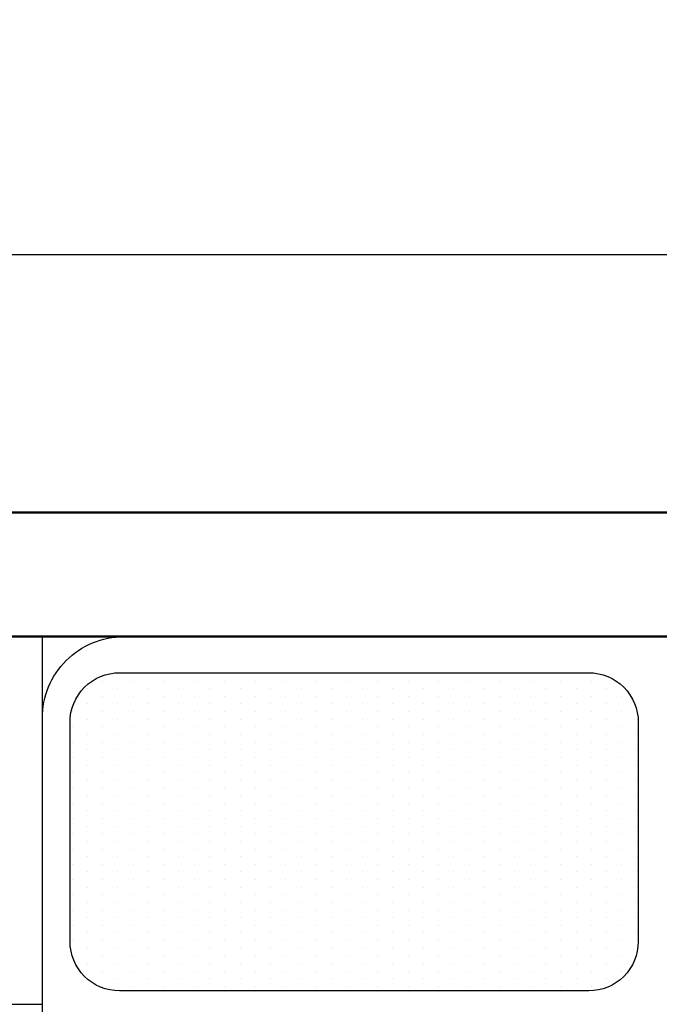
# Model space of a CAD drawing. Units: inches. Extents: x 3064 to 19385, y 846 to 15425.
# Tile 22 of 108: x 3855 to 3886, y 1373 to 1420. Entities that reach past the tile are written whole.
import ezdxf

# ---------------------------------------------------------------- set-up
doc = ezdxf.new("R2010")
doc.units = ezdxf.units.IN
for name, color, linetype, lineweight in [('A-ANNO-DIMS', 2, 'Continuous', 18), ('A-FLOR-FIXT', 9, 'Continuous', 18), ('A-WALL', 7, 'Continuous', 50)]:
    doc.layers.add(name, color=color, linetype=linetype, lineweight=lineweight)
doc.layers.add('BLOCK', color=6, linetype='Continuous')
doc.styles.get("Standard").update_dxf_attribs({"font": 'arial.ttf'})
doc.dimstyles.new('ISO-25', dxfattribs={"dimtxt": 9, "dimasz": 2.5, "dimexe": 1.25, "dimexo": 0.625, "dimtad": 1, "dimdec": 1, "dimlunit": 3, "dimtxsty": 'Standard', "dimcen": 2.5, "dimadec": 0, "dimazin": 0, "dimtfac": 1, "dimtdec": 1, "dimtmove": 0, "dimatfit": 3, "dimfxl": 1, "dimarcsym": 0})

# ---------------------------------------------------------------- blocks, each defined once
blk = doc.blocks.new('*X7')
at = {"color": 0}
for p, q in [((266.4375, 457.03125), (266.4375, 457.03125)), ((266.8125, 457.03125), (266.8125, 457.03125)), ((267.1875, 457.03125), (267.1875, 457.03125)), ((267.5625, 457.03125), (267.5625, 457.03125)), ((267.9375, 457.03125), (267.9375, 457.03125)), ((268.3125, 457.03125), (268.3125, 457.03125)), ((268.6875, 457.03125), (268.6875, 457.03125)), ((269.0625, 457.03125), (269.0625, 457.03125)), ((269.4375, 457.03125), (269.4375, 457.03125)), ((269.8125, 457.03125), (269.8125, 457.03125)), ((270.1875, 457.03125), (270.1875, 457.03125)), ((270.5625, 457.03125), (270.5625, 457.03125)), ((270.9375, 457.03125), (270.9375, 457.03125)), ((271.3125, 457.03125), (271.3125, 457.03125)), ((271.6875, 457.03125), (271.6875, 457.03125)), ((272.0625, 457.03125), (272.0625, 457.03125)), ((266.0625, 456.84375), (266.0625, 456.84375)), ((266.25, 456.9375), (266.25, 456.9375)), ((266.4375, 456.84375), (266.4375, 456.84375)), ((266.625, 456.9375), (266.625, 456.9375)), ((266.8125, 456.84375), (266.8125, 456.84375)), ((267, 456.9375), (267, 456.9375)), ((267.1875, 456.84375), (267.1875, 456.84375)), ((267.375, 456.9375), (267.375, 456.9375)), ((267.5625, 456.84375), (267.5625, 456.84375)), ((267.75, 456.9375), (267.75, 456.9375)), ((267.9375, 456.84375), (267.9375, 456.84375)), ((268.125, 456.9375), (268.125, 456.9375)), ((268.3125, 456.84375), (268.3125, 456.84375)), ((268.5, 456.9375), (268.5, 456.9375)), ((268.6875, 456.84375), (268.6875, 456.84375)), ((268.875, 456.9375), (268.875, 456.9375)), ((269.0625, 456.84375), (269.0625, 456.84375)), ((269.25, 456.9375), (269.25, 456.9375)), ((269.4375, 456.84375), (269.4375, 456.84375)), ((269.625, 456.9375), (269.625, 456.9375)), ((269.8125, 456.84375), (269.8125, 456.84375)), ((270, 456.9375), (270, 456.9375)), ((270.1875, 456.84375), (270.1875, 456.84375)), ((270.375, 456.9375), (270.375, 456.9375)), ((270.5625, 456.84375), (270.5625, 456.84375)), ((270.75, 456.9375), (270.75, 456.9375)), ((270.9375, 456.84375), (270.9375, 456.84375)), ((271.125, 456.9375), (271.125, 456.9375)), ((271.3125, 456.84375), (271.3125, 456.84375)), ((271.5, 456.9375), (271.5, 456.9375)), ((271.6875, 456.84375), (271.6875, 456.84375)), ((271.875, 456.9375), (271.875, 456.9375)), ((272.0625, 456.84375), (272.0625, 456.84375)), ((272.25, 456.9375), (272.25, 456.9375)), ((272.4375, 456.84375), (272.4375, 456.84375)), ((266.25, 456.75), (266.25, 456.75)), ((266.625, 456.75), (266.625, 456.75)), ((267, 456.75), (267, 456.75)), ((267.375, 456.75), (267.375, 456.75)), ((267.75, 456.75), (267.75, 456.75)), ((268.125, 456.75), (268.125, 456.75)), ((268.5, 456.75), (268.5, 456.75)), ((268.875, 456.75), (268.875, 456.75)), ((269.25, 456.75), (269.25, 456.75)), ((269.625, 456.75), (269.625, 456.75)), ((270, 456.75), (270, 456.75)), ((270.375, 456.75), (270.375, 456.75)), ((270.75, 456.75), (270.75, 456.75)), ((271.125, 456.75), (271.125, 456.75)), ((271.5, 456.75), (271.5, 456.75)), ((271.875, 456.75), (271.875, 456.75)), ((272.25, 456.75), (272.25, 456.75)), ((272.625, 456.75), (272.625, 456.75)), ((266.0625, 456.65625), (266.0625, 456.65625)), ((266.4375, 456.65625), (266.4375, 456.65625)), ((266.8125, 456.65625), (266.8125, 456.65625)), ((267.1875, 456.65625), (267.1875, 456.65625)), ((267.5625, 456.65625), (267.5625, 456.65625)), ((267.9375, 456.65625), (267.9375, 456.65625)), ((268.3125, 456.65625), (268.3125, 456.65625)), ((268.6875, 456.65625), (268.6875, 456.65625)), ((269.0625, 456.65625), (269.0625, 456.65625)), ((269.4375, 456.65625), (269.4375, 456.65625)), ((269.8125, 456.65625), (269.8125, 456.65625)), ((270.1875, 456.65625), (270.1875, 456.65625)), ((270.5625, 456.65625), (270.5625, 456.65625)), ((270.9375, 456.65625), (270.9375, 456.65625)), ((271.3125, 456.65625), (271.3125, 456.65625)), ((271.6875, 456.65625), (271.6875, 456.65625)), ((272.0625, 456.65625), (272.0625, 456.65625)), ((272.4375, 456.65625), (272.4375, 456.65625)), ((265.875, 456.5625), (265.875, 456.5625)), ((266.25, 456.5625), (266.25, 456.5625)), ((266.625, 456.5625), (266.625, 456.5625)), ((267, 456.5625), (267, 456.5625)), ((267.375, 456.5625), (267.375, 456.5625)), ((267.75, 456.5625), (267.75, 456.5625)), ((268.125, 456.5625), (268.125, 456.5625)), ((268.5, 456.5625), (268.5, 456.5625)), ((268.875, 456.5625), (268.875, 456.5625)), ((269.25, 456.5625), (269.25, 456.5625)), ((269.625, 456.5625), (269.625, 456.5625)), ((270, 456.5625), (270, 456.5625)), ((270.375, 456.5625), (270.375, 456.5625)), ((270.75, 456.5625), (270.75, 456.5625)), ((271.125, 456.5625), (271.125, 456.5625)), ((271.5, 456.5625), (271.5, 456.5625)), ((271.875, 456.5625), (271.875, 456.5625)), ((272.25, 456.5625), (272.25, 456.5625)), ((272.625, 456.5625), (272.625, 456.5625)), ((265.875, 456.375), (265.875, 456.375)), ((266.0625, 456.46875), (266.0625, 456.46875)), ((266.25, 456.375), (266.25, 456.375)), ((266.4375, 456.46875), (266.4375, 456.46875)), ((266.625, 456.375), (266.625, 456.375)), ((266.8125, 456.46875), (266.8125, 456.46875)), ((267, 456.375), (267, 456.375)), ((267.1875, 456.46875), (267.1875, 456.46875)), ((267.375, 456.375), (267.375, 456.375)), ((267.5625, 456.46875), (267.5625, 456.46875)), ((267.75, 456.375), (267.75, 456.375)), ((267.9375, 456.46875), (267.9375, 456.46875)), ((268.125, 456.375), (268.125, 456.375)), ((268.3125, 456.46875), (268.3125, 456.46875)), ((268.5, 456.375), (268.5, 456.375)), ((268.6875, 456.46875), (268.6875, 456.46875)), ((268.875, 456.375), (268.875, 456.375)), ((269.0625, 456.46875), (269.0625, 456.46875)), ((269.25, 456.375), (269.25, 456.375)), ((269.4375, 456.46875), (269.4375, 456.46875)), ((269.625, 456.375), (269.625, 456.375)), ((269.8125, 456.46875), (269.8125, 456.46875)), ((270, 456.375), (270, 456.375)), ((270.1875, 456.46875), (270.1875, 456.46875)), ((270.375, 456.375), (270.375, 456.375)), ((270.5625, 456.46875), (270.5625, 456.46875)), ((270.75, 456.375), (270.75, 456.375)), ((270.9375, 456.46875), (270.9375, 456.46875)), ((271.125, 456.375), (271.125, 456.375)), ((271.3125, 456.46875), (271.3125, 456.46875)), ((271.5, 456.375), (271.5, 456.375)), ((271.6875, 456.46875), (271.6875, 456.46875)), ((271.875, 456.375), (271.875, 456.375)), ((272.0625, 456.46875), (272.0625, 456.46875)), ((272.25, 456.375), (272.25, 456.375)), ((272.4375, 456.46875), (272.4375, 456.46875)), ((272.625, 456.375), (272.625, 456.375)), ((272.8125, 456.46875), (272.8125, 456.46875)), ((266.0625, 456.28125), (266.0625, 456.28125)), ((266.4375, 456.28125), (266.4375, 456.28125)), ((266.8125, 456.28125), (266.8125, 456.28125)), ((267.1875, 456.28125), (267.1875, 456.28125)), ((267.5625, 456.28125), (267.5625, 456.28125)), ((267.9375, 456.28125), (267.9375, 456.28125)), ((268.3125, 456.28125), (268.3125, 456.28125)), ((268.6875, 456.28125), (268.6875, 456.28125)), ((269.0625, 456.28125), (269.0625, 456.28125)), ((269.4375, 456.28125), (269.4375, 456.28125)), ((269.8125, 456.28125), (269.8125, 456.28125)), ((270.1875, 456.28125), (270.1875, 456.28125)), ((270.5625, 456.28125), (270.5625, 456.28125)), ((270.9375, 456.28125), (270.9375, 456.28125)), ((271.3125, 456.28125), (271.3125, 456.28125)), ((271.6875, 456.28125), (271.6875, 456.28125)), ((272.0625, 456.28125), (272.0625, 456.28125)), ((272.4375, 456.28125), (272.4375, 456.28125)), ((272.8125, 456.28125), (272.8125, 456.28125)), ((265.875, 456.1875), (265.875, 456.1875)), ((266.25, 456.1875), (266.25, 456.1875)), ((266.625, 456.1875), (266.625, 456.1875)), ((267, 456.1875), (267, 456.1875)), ((267.375, 456.1875), (267.375, 456.1875)), ((267.75, 456.1875), (267.75, 456.1875)), ((268.125, 456.1875), (268.125, 456.1875)), ((268.5, 456.1875), (268.5, 456.1875)), ((268.875, 456.1875), (268.875, 456.1875)), ((269.25, 456.1875), (269.25, 456.1875)), ((269.625, 456.1875), (269.625, 456.1875)), ((270, 456.1875), (270, 456.1875)), ((270.375, 456.1875), (270.375, 456.1875)), ((270.75, 456.1875), (270.75, 456.1875)), ((271.125, 456.1875), (271.125, 456.1875)), ((271.5, 456.1875), (271.5, 456.1875)), ((271.875, 456.1875), (271.875, 456.1875)), ((272.25, 456.1875), (272.25, 456.1875)), ((272.625, 456.1875), (272.625, 456.1875)), ((265.875, 456), (265.875, 456)), ((266.0625, 456.09375), (266.0625, 456.09375)), ((266.25, 456), (266.25, 456)), ((266.4375, 456.09375), (266.4375, 456.09375)), ((266.625, 456), (266.625, 456)), ((266.8125, 456.09375), (266.8125, 456.09375)), ((267, 456), (267, 456)), ((267.1875, 456.09375), (267.1875, 456.09375)), ((267.375, 456), (267.375, 456)), ((267.5625, 456.09375), (267.5625, 456.09375)), ((267.75, 456), (267.75, 456)), ((267.9375, 456.09375), (267.9375, 456.09375)), ((268.125, 456), (268.125, 456)), ((268.3125, 456.09375), (268.3125, 456.09375)), ((268.5, 456), (268.5, 456)), ((268.6875, 456.09375), (268.6875, 456.09375)), ((268.875, 456), (268.875, 456)), ((269.0625, 456.09375), (269.0625, 456.09375)), ((269.25, 456), (269.25, 456)), ((269.4375, 456.09375), (269.4375, 456.09375)), ((269.625, 456), (269.625, 456)), ((269.8125, 456.09375), (269.8125, 456.09375)), ((270, 456), (270, 456)), ((270.1875, 456.09375), (270.1875, 456.09375)), ((270.375, 456), (270.375, 456)), ((270.5625, 456.09375), (270.5625, 456.09375)), ((270.75, 456), (270.75, 456)), ((270.9375, 456.09375), (270.9375, 456.09375)), ((271.125, 456), (271.125, 456)), ((271.3125, 456.09375), (271.3125, 456.09375)), ((271.5, 456), (271.5, 456)), ((271.6875, 456.09375), (271.6875, 456.09375)), ((271.875, 456), (271.875, 456)), ((272.0625, 456.09375), (272.0625, 456.09375)), ((272.25, 456), (272.25, 456)), ((272.4375, 456.09375), (272.4375, 456.09375)), ((272.625, 456), (272.625, 456)), ((272.8125, 456.09375), (272.8125, 456.09375)), ((266.0625, 455.90625), (266.0625, 455.90625)), ((266.4375, 455.90625), (266.4375, 455.90625)), ((266.8125, 455.90625), (266.8125, 455.90625)), ((267.1875, 455.90625), (267.1875, 455.90625)), ((267.5625, 455.90625), (267.5625, 455.90625)), ((267.9375, 455.90625), (267.9375, 455.90625)), ((268.3125, 455.90625), (268.3125, 455.90625)), ((268.6875, 455.90625), (268.6875, 455.90625)), ((269.0625, 455.90625), (269.0625, 455.90625)), ((269.4375, 455.90625), (269.4375, 455.90625)), ((269.8125, 455.90625), (269.8125, 455.90625)), ((270.1875, 455.90625), (270.1875, 455.90625)), ((270.5625, 455.90625), (270.5625, 455.90625)), ((270.9375, 455.90625), (270.9375, 455.90625)), ((271.3125, 455.90625), (271.3125, 455.90625)), ((271.6875, 455.90625), (271.6875, 455.90625)), ((272.0625, 455.90625), (272.0625, 455.90625)), ((272.4375, 455.90625), (272.4375, 455.90625)), ((272.8125, 455.90625), (272.8125, 455.90625)), ((265.875, 455.8125), (265.875, 455.8125)), ((266.25, 455.8125), (266.25, 455.8125)), ((266.625, 455.8125), (266.625, 455.8125)), ((267, 455.8125), (267, 455.8125)), ((267.375, 455.8125), (267.375, 455.8125)), ((267.75, 455.8125), (267.75, 455.8125)), ((268.125, 455.8125), (268.125, 455.8125)), ((268.5, 455.8125), (268.5, 455.8125)), ((268.875, 455.8125), (268.875, 455.8125)), ((269.25, 455.8125), (269.25, 455.8125)), ((269.625, 455.8125), (269.625, 455.8125)), ((270, 455.8125), (270, 455.8125)), ((270.375, 455.8125), (270.375, 455.8125)), ((270.75, 455.8125), (270.75, 455.8125)), ((271.125, 455.8125), (271.125, 455.8125)), ((271.5, 455.8125), (271.5, 455.8125)), ((271.875, 455.8125), (271.875, 455.8125)), ((272.25, 455.8125), (272.25, 455.8125)), ((272.625, 455.8125), (272.625, 455.8125)), ((265.875, 455.625), (265.875, 455.625)), ((266.0625, 455.71875), (266.0625, 455.71875)), ((266.25, 455.625), (266.25, 455.625)), ((266.4375, 455.71875), (266.4375, 455.71875)), ((266.625, 455.625), (266.625, 455.625)), ((266.8125, 455.71875), (266.8125, 455.71875)), ((267, 455.625), (267, 455.625)), ((267.1875, 455.71875), (267.1875, 455.71875)), ((267.375, 455.625), (267.375, 455.625)), ((267.5625, 455.71875), (267.5625, 455.71875)), ((267.75, 455.625), (267.75, 455.625)), ((267.9375, 455.71875), (267.9375, 455.71875)), ((268.125, 455.625), (268.125, 455.625)), ((268.3125, 455.71875), (268.3125, 455.71875)), ((268.5, 455.625), (268.5, 455.625)), ((268.6875, 455.71875), (268.6875, 455.71875)), ((268.875, 455.625), (268.875, 455.625)), ((269.0625, 455.71875), (269.0625, 455.71875)), ((269.25, 455.625), (269.25, 455.625)), ((269.4375, 455.71875), (269.4375, 455.71875)), ((269.625, 455.625), (269.625, 455.625)), ((269.8125, 455.71875), (269.8125, 455.71875)), ((270, 455.625), (270, 455.625)), ((270.1875, 455.71875), (270.1875, 455.71875)), ((270.375, 455.625), (270.375, 455.625)), ((270.5625, 455.71875), (270.5625, 455.71875)), ((270.75, 455.625), (270.75, 455.625)), ((270.9375, 455.71875), (270.9375, 455.71875)), ((271.125, 455.625), (271.125, 455.625)), ((271.3125, 455.71875), (271.3125, 455.71875)), ((271.5, 455.625), (271.5, 455.625)), ((271.6875, 455.71875), (271.6875, 455.71875)), ((271.875, 455.625), (271.875, 455.625)), ((272.0625, 455.71875), (272.0625, 455.71875)), ((272.25, 455.625), (272.25, 455.625)), ((272.4375, 455.71875), (272.4375, 455.71875)), ((272.625, 455.625), (272.625, 455.625)), ((272.8125, 455.71875), (272.8125, 455.71875)), ((266.0625, 455.53125), (266.0625, 455.53125)), ((266.4375, 455.53125), (266.4375, 455.53125)), ((266.8125, 455.53125), (266.8125, 455.53125)), ((267.1875, 455.53125), (267.1875, 455.53125)), ((267.5625, 455.53125), (267.5625, 455.53125)), ((267.9375, 455.53125), (267.9375, 455.53125)), ((268.3125, 455.53125), (268.3125, 455.53125)), ((268.6875, 455.53125), (268.6875, 455.53125)), ((269.0625, 455.53125), (269.0625, 455.53125)), ((269.4375, 455.53125), (269.4375, 455.53125)), ((269.8125, 455.53125), (269.8125, 455.53125)), ((270.1875, 455.53125), (270.1875, 455.53125)), ((270.5625, 455.53125), (270.5625, 455.53125)), ((270.9375, 455.53125), (270.9375, 455.53125)), ((271.3125, 455.53125), (271.3125, 455.53125)), ((271.6875, 455.53125), (271.6875, 455.53125)), ((272.0625, 455.53125), (272.0625, 455.53125)), ((272.4375, 455.53125), (272.4375, 455.53125)), ((272.8125, 455.53125), (272.8125, 455.53125)), ((265.875, 455.4375), (265.875, 455.4375)), ((266.25, 455.4375), (266.25, 455.4375)), ((266.625, 455.4375), (266.625, 455.4375)), ((267, 455.4375), (267, 455.4375)), ((267.375, 455.4375), (267.375, 455.4375)), ((267.75, 455.4375), (267.75, 455.4375)), ((268.125, 455.4375), (268.125, 455.4375)), ((268.5, 455.4375), (268.5, 455.4375)), ((268.875, 455.4375), (268.875, 455.4375)), ((269.25, 455.4375), (269.25, 455.4375)), ((269.625, 455.4375), (269.625, 455.4375)), ((270, 455.4375), (270, 455.4375)), ((270.375, 455.4375), (270.375, 455.4375)), ((270.75, 455.4375), (270.75, 455.4375)), ((271.125, 455.4375), (271.125, 455.4375)), ((271.5, 455.4375), (271.5, 455.4375)), ((271.875, 455.4375), (271.875, 455.4375)), ((272.25, 455.4375), (272.25, 455.4375)), ((272.625, 455.4375), (272.625, 455.4375)), ((266.0625, 455.34375), (266.0625, 455.34375)), ((266.4375, 455.34375), (266.4375, 455.34375)), ((266.8125, 455.34375), (266.8125, 455.34375)), ((267.1875, 455.34375), (267.1875, 455.34375)), ((267.5625, 455.34375), (267.5625, 455.34375)), ((267.9375, 455.34375), (267.9375, 455.34375)), ((268.3125, 455.34375), (268.3125, 455.34375)), ((268.6875, 455.34375), (268.6875, 455.34375)), ((269.0625, 455.34375), (269.0625, 455.34375)), ((269.4375, 455.34375), (269.4375, 455.34375)), ((269.8125, 455.34375), (269.8125, 455.34375)), ((270.1875, 455.34375), (270.1875, 455.34375)), ((270.5625, 455.34375), (270.5625, 455.34375)), ((270.9375, 455.34375), (270.9375, 455.34375)), ((271.3125, 455.34375), (271.3125, 455.34375)), ((271.6875, 455.34375), (271.6875, 455.34375)), ((272.0625, 455.34375), (272.0625, 455.34375)), ((272.4375, 455.34375), (272.4375, 455.34375)), ((272.8125, 455.34375), (272.8125, 455.34375)), ((265.875, 455.25), (265.875, 455.25)), ((266.0625, 455.15625), (266.0625, 455.15625)), ((266.25, 455.25), (266.25, 455.25)), ((266.4375, 455.15625), (266.4375, 455.15625)), ((266.625, 455.25), (266.625, 455.25)), ((266.8125, 455.15625), (266.8125, 455.15625)), ((267, 455.25), (267, 455.25)), ((267.1875, 455.15625), (267.1875, 455.15625)), ((267.375, 455.25), (267.375, 455.25)), ((267.5625, 455.15625), (267.5625, 455.15625)), ((267.75, 455.25), (267.75, 455.25)), ((267.9375, 455.15625), (267.9375, 455.15625)), ((268.125, 455.25), (268.125, 455.25)), ((268.3125, 455.15625), (268.3125, 455.15625)), ((268.5, 455.25), (268.5, 455.25)), ((268.6875, 455.15625), (268.6875, 455.15625)), ((268.875, 455.25), (268.875, 455.25)), ((269.0625, 455.15625), (269.0625, 455.15625)), ((269.25, 455.25), (269.25, 455.25)), ((269.4375, 455.15625), (269.4375, 455.15625)), ((269.625, 455.25), (269.625, 455.25)), ((269.8125, 455.15625), (269.8125, 455.15625)), ((270, 455.25), (270, 455.25)), ((270.1875, 455.15625), (270.1875, 455.15625)), ((270.375, 455.25), (270.375, 455.25)), ((270.5625, 455.15625), (270.5625, 455.15625)), ((270.75, 455.25), (270.75, 455.25)), ((270.9375, 455.15625), (270.9375, 455.15625)), ((271.125, 455.25), (271.125, 455.25)), ((271.3125, 455.15625), (271.3125, 455.15625)), ((271.5, 455.25), (271.5, 455.25)), ((271.6875, 455.15625), (271.6875, 455.15625)), ((271.875, 455.25), (271.875, 455.25)), ((272.0625, 455.15625), (272.0625, 455.15625)), ((272.25, 455.25), (272.25, 455.25)), ((272.4375, 455.15625), (272.4375, 455.15625)), ((272.625, 455.25), (272.625, 455.25)), ((272.8125, 455.15625), (272.8125, 455.15625)), ((265.875, 455.0625), (265.875, 455.0625)), ((266.25, 455.0625), (266.25, 455.0625)), ((266.625, 455.0625), (266.625, 455.0625)), ((267, 455.0625), (267, 455.0625)), ((267.375, 455.0625), (267.375, 455.0625)), ((267.75, 455.0625), (267.75, 455.0625)), ((268.125, 455.0625), (268.125, 455.0625)), ((268.5, 455.0625), (268.5, 455.0625)), ((268.875, 455.0625), (268.875, 455.0625)), ((269.25, 455.0625), (269.25, 455.0625)), ((269.625, 455.0625), (269.625, 455.0625)), ((270, 455.0625), (270, 455.0625)), ((270.375, 455.0625), (270.375, 455.0625)), ((270.75, 455.0625), (270.75, 455.0625)), ((271.125, 455.0625), (271.125, 455.0625)), ((271.5, 455.0625), (271.5, 455.0625)), ((271.875, 455.0625), (271.875, 455.0625)), ((272.25, 455.0625), (272.25, 455.0625)), ((272.625, 455.0625), (272.625, 455.0625)), ((266.0625, 454.96875), (266.0625, 454.96875)), ((266.4375, 454.96875), (266.4375, 454.96875)), ((266.8125, 454.96875), (266.8125, 454.96875)), ((267.1875, 454.96875), (267.1875, 454.96875)), ((267.5625, 454.96875), (267.5625, 454.96875)), ((267.9375, 454.96875), (267.9375, 454.96875)), ((268.3125, 454.96875), (268.3125, 454.96875)), ((268.6875, 454.96875), (268.6875, 454.96875)), ((269.0625, 454.96875), (269.0625, 454.96875)), ((269.4375, 454.96875), (269.4375, 454.96875)), ((269.8125, 454.96875), (269.8125, 454.96875)), ((270.1875, 454.96875), (270.1875, 454.96875)), ((270.5625, 454.96875), (270.5625, 454.96875)), ((270.9375, 454.96875), (270.9375, 454.96875)), ((271.3125, 454.96875), (271.3125, 454.96875)), ((271.6875, 454.96875), (271.6875, 454.96875)), ((272.0625, 454.96875), (272.0625, 454.96875)), ((272.4375, 454.96875), (272.4375, 454.96875)), ((272.8125, 454.96875), (272.8125, 454.96875)), ((265.875, 454.875), (265.875, 454.875)), ((266.0625, 454.78125), (266.0625, 454.78125)), ((266.25, 454.875), (266.25, 454.875)), ((266.4375, 454.78125), (266.4375, 454.78125)), ((266.625, 454.875), (266.625, 454.875)), ((266.8125, 454.78125), (266.8125, 454.78125)), ((267, 454.875), (267, 454.875)), ((267.1875, 454.78125), (267.1875, 454.78125)), ((267.375, 454.875), (267.375, 454.875)), ((267.5625, 454.78125), (267.5625, 454.78125)), ((267.75, 454.875), (267.75, 454.875)), ((267.9375, 454.78125), (267.9375, 454.78125)), ((268.125, 454.875), (268.125, 454.875)), ((268.3125, 454.78125), (268.3125, 454.78125)), ((268.5, 454.875), (268.5, 454.875)), ((268.6875, 454.78125), (268.6875, 454.78125)), ((268.875, 454.875), (268.875, 454.875)), ((269.0625, 454.78125), (269.0625, 454.78125)), ((269.25, 454.875), (269.25, 454.875)), ((269.4375, 454.78125), (269.4375, 454.78125)), ((269.625, 454.875), (269.625, 454.875)), ((269.8125, 454.78125), (269.8125, 454.78125)), ((270, 454.875), (270, 454.875)), ((270.1875, 454.78125), (270.1875, 454.78125)), ((270.375, 454.875), (270.375, 454.875)), ((270.5625, 454.78125), (270.5625, 454.78125)), ((270.75, 454.875), (270.75, 454.875)), ((270.9375, 454.78125), (270.9375, 454.78125)), ((271.125, 454.875), (271.125, 454.875)), ((271.3125, 454.78125), (271.3125, 454.78125)), ((271.5, 454.875), (271.5, 454.875)), ((271.6875, 454.78125), (271.6875, 454.78125)), ((271.875, 454.875), (271.875, 454.875)), ((272.0625, 454.78125), (272.0625, 454.78125)), ((272.25, 454.875), (272.25, 454.875)), ((272.4375, 454.78125), (272.4375, 454.78125)), ((272.625, 454.875), (272.625, 454.875)), ((272.8125, 454.78125), (272.8125, 454.78125)), ((265.875, 454.6875), (265.875, 454.6875)), ((266.25, 454.6875), (266.25, 454.6875)), ((266.625, 454.6875), (266.625, 454.6875)), ((267, 454.6875), (267, 454.6875)), ((267.375, 454.6875), (267.375, 454.6875)), ((267.75, 454.6875), (267.75, 454.6875)), ((268.125, 454.6875), (268.125, 454.6875)), ((268.5, 454.6875), (268.5, 454.6875)), ((268.875, 454.6875), (268.875, 454.6875)), ((269.25, 454.6875), (269.25, 454.6875)), ((269.625, 454.6875), (269.625, 454.6875)), ((270, 454.6875), (270, 454.6875)), ((270.375, 454.6875), (270.375, 454.6875)), ((270.75, 454.6875), (270.75, 454.6875)), ((271.125, 454.6875), (271.125, 454.6875)), ((271.5, 454.6875), (271.5, 454.6875)), ((271.875, 454.6875), (271.875, 454.6875)), ((272.25, 454.6875), (272.25, 454.6875)), ((272.625, 454.6875), (272.625, 454.6875)), ((266.0625, 454.59375), (266.0625, 454.59375)), ((266.4375, 454.59375), (266.4375, 454.59375)), ((266.8125, 454.59375), (266.8125, 454.59375)), ((267.1875, 454.59375), (267.1875, 454.59375)), ((267.5625, 454.59375), (267.5625, 454.59375)), ((267.9375, 454.59375), (267.9375, 454.59375)), ((268.3125, 454.59375), (268.3125, 454.59375)), ((268.6875, 454.59375), (268.6875, 454.59375)), ((269.0625, 454.59375), (269.0625, 454.59375)), ((269.4375, 454.59375), (269.4375, 454.59375)), ((269.8125, 454.59375), (269.8125, 454.59375)), ((270.1875, 454.59375), (270.1875, 454.59375)), ((270.5625, 454.59375), (270.5625, 454.59375)), ((270.9375, 454.59375), (270.9375, 454.59375)), ((271.3125, 454.59375), (271.3125, 454.59375)), ((271.6875, 454.59375), (271.6875, 454.59375)), ((272.0625, 454.59375), (272.0625, 454.59375)), ((272.4375, 454.59375), (272.4375, 454.59375)), ((272.8125, 454.59375), (272.8125, 454.59375)), ((265.875, 454.5), (265.875, 454.5)), ((266.25, 454.5), (266.25, 454.5)), ((266.625, 454.5), (266.625, 454.5)), ((267, 454.5), (267, 454.5)), ((267.375, 454.5), (267.375, 454.5)), ((267.75, 454.5), (267.75, 454.5)), ((268.125, 454.5), (268.125, 454.5)), ((268.5, 454.5), (268.5, 454.5)), ((268.875, 454.5), (268.875, 454.5)), ((269.25, 454.5), (269.25, 454.5)), ((269.625, 454.5), (269.625, 454.5)), ((270, 454.5), (270, 454.5)), ((270.375, 454.5), (270.375, 454.5)), ((270.75, 454.5), (270.75, 454.5)), ((271.125, 454.5), (271.125, 454.5)), ((271.5, 454.5), (271.5, 454.5)), ((271.875, 454.5), (271.875, 454.5)), ((272.25, 454.5), (272.25, 454.5)), ((272.625, 454.5), (272.625, 454.5)), ((265.875, 454.3125), (265.875, 454.3125)), ((266.0625, 454.40625), (266.0625, 454.40625)), ((266.25, 454.3125), (266.25, 454.3125)), ((266.4375, 454.40625), (266.4375, 454.40625)), ((266.625, 454.3125), (266.625, 454.3125)), ((266.8125, 454.40625), (266.8125, 454.40625)), ((267, 454.3125), (267, 454.3125)), ((267.1875, 454.40625), (267.1875, 454.40625)), ((267.375, 454.3125), (267.375, 454.3125)), ((267.5625, 454.40625), (267.5625, 454.40625)), ((267.75, 454.3125), (267.75, 454.3125)), ((267.9375, 454.40625), (267.9375, 454.40625)), ((268.125, 454.3125), (268.125, 454.3125)), ((268.3125, 454.40625), (268.3125, 454.40625)), ((268.5, 454.3125), (268.5, 454.3125)), ((268.6875, 454.40625), (268.6875, 454.40625)), ((268.875, 454.3125), (268.875, 454.3125)), ((269.0625, 454.40625), (269.0625, 454.40625)), ((269.25, 454.3125), (269.25, 454.3125)), ((269.4375, 454.40625), (269.4375, 454.40625)), ((269.625, 454.3125), (269.625, 454.3125)), ((269.8125, 454.40625), (269.8125, 454.40625)), ((270, 454.3125), (270, 454.3125)), ((270.1875, 454.40625), (270.1875, 454.40625)), ((270.375, 454.3125), (270.375, 454.3125)), ((270.5625, 454.40625), (270.5625, 454.40625)), ((270.75, 454.3125), (270.75, 454.3125)), ((270.9375, 454.40625), (270.9375, 454.40625)), ((271.125, 454.3125), (271.125, 454.3125)), ((271.3125, 454.40625), (271.3125, 454.40625)), ((271.5, 454.3125), (271.5, 454.3125)), ((271.6875, 454.40625), (271.6875, 454.40625)), ((271.875, 454.3125), (271.875, 454.3125)), ((272.0625, 454.40625), (272.0625, 454.40625)), ((272.25, 454.3125), (272.25, 454.3125)), ((272.4375, 454.40625), (272.4375, 454.40625)), ((272.625, 454.3125), (272.625, 454.3125)), ((272.8125, 454.40625), (272.8125, 454.40625)), ((266.0625, 454.21875), (266.0625, 454.21875)), ((266.4375, 454.21875), (266.4375, 454.21875)), ((266.8125, 454.21875), (266.8125, 454.21875)), ((267.1875, 454.21875), (267.1875, 454.21875)), ((267.5625, 454.21875), (267.5625, 454.21875)), ((267.9375, 454.21875), (267.9375, 454.21875)), ((268.3125, 454.21875), (268.3125, 454.21875)), ((268.6875, 454.21875), (268.6875, 454.21875)), ((269.0625, 454.21875), (269.0625, 454.21875)), ((269.4375, 454.21875), (269.4375, 454.21875)), ((269.8125, 454.21875), (269.8125, 454.21875)), ((270.1875, 454.21875), (270.1875, 454.21875)), ((270.5625, 454.21875), (270.5625, 454.21875)), ((270.9375, 454.21875), (270.9375, 454.21875)), ((271.3125, 454.21875), (271.3125, 454.21875)), ((271.6875, 454.21875), (271.6875, 454.21875)), ((272.0625, 454.21875), (272.0625, 454.21875)), ((272.4375, 454.21875), (272.4375, 454.21875)), ((272.8125, 454.21875), (272.8125, 454.21875)), ((265.875, 454.125), (265.875, 454.125)), ((266.25, 454.125), (266.25, 454.125)), ((266.625, 454.125), (266.625, 454.125)), ((267, 454.125), (267, 454.125)), ((267.375, 454.125), (267.375, 454.125)), ((267.75, 454.125), (267.75, 454.125)), ((268.125, 454.125), (268.125, 454.125)), ((268.5, 454.125), (268.5, 454.125)), ((268.875, 454.125), (268.875, 454.125)), ((269.25, 454.125), (269.25, 454.125)), ((269.625, 454.125), (269.625, 454.125)), ((270, 454.125), (270, 454.125)), ((270.375, 454.125), (270.375, 454.125)), ((270.75, 454.125), (270.75, 454.125)), ((271.125, 454.125), (271.125, 454.125)), ((271.5, 454.125), (271.5, 454.125)), ((271.875, 454.125), (271.875, 454.125)), ((272.25, 454.125), (272.25, 454.125)), ((272.625, 454.125), (272.625, 454.125)), ((265.875, 453.9375), (265.875, 453.9375)), ((266.0625, 454.03125), (266.0625, 454.03125)), ((266.25, 453.9375), (266.25, 453.9375)), ((266.4375, 454.03125), (266.4375, 454.03125)), ((266.625, 453.9375), (266.625, 453.9375)), ((266.8125, 454.03125), (266.8125, 454.03125)), ((267, 453.9375), (267, 453.9375)), ((267.1875, 454.03125), (267.1875, 454.03125)), ((267.375, 453.9375), (267.375, 453.9375)), ((267.5625, 454.03125), (267.5625, 454.03125)), ((267.75, 453.9375), (267.75, 453.9375)), ((267.9375, 454.03125), (267.9375, 454.03125)), ((268.125, 453.9375), (268.125, 453.9375)), ((268.3125, 454.03125), (268.3125, 454.03125)), ((268.5, 453.9375), (268.5, 453.9375)), ((268.6875, 454.03125), (268.6875, 454.03125)), ((268.875, 453.9375), (268.875, 453.9375)), ((269.0625, 454.03125), (269.0625, 454.03125)), ((269.25, 453.9375), (269.25, 453.9375)), ((269.4375, 454.03125), (269.4375, 454.03125)), ((269.625, 453.9375), (269.625, 453.9375)), ((269.8125, 454.03125), (269.8125, 454.03125)), ((270, 453.9375), (270, 453.9375)), ((270.1875, 454.03125), (270.1875, 454.03125)), ((270.375, 453.9375), (270.375, 453.9375)), ((270.5625, 454.03125), (270.5625, 454.03125)), ((270.75, 453.9375), (270.75, 453.9375)), ((270.9375, 454.03125), (270.9375, 454.03125)), ((271.125, 453.9375), (271.125, 453.9375)), ((271.3125, 454.03125), (271.3125, 454.03125)), ((271.5, 453.9375), (271.5, 453.9375)), ((271.6875, 454.03125), (271.6875, 454.03125)), ((271.875, 453.9375), (271.875, 453.9375)), ((272.0625, 454.03125), (272.0625, 454.03125)), ((272.25, 453.9375), (272.25, 453.9375)), ((272.4375, 454.03125), (272.4375, 454.03125)), ((272.625, 453.9375), (272.625, 453.9375)), ((272.8125, 454.03125), (272.8125, 454.03125)), ((266.0625, 453.84375), (266.0625, 453.84375)), ((266.4375, 453.84375), (266.4375, 453.84375)), ((266.8125, 453.84375), (266.8125, 453.84375)), ((267.1875, 453.84375), (267.1875, 453.84375)), ((267.5625, 453.84375), (267.5625, 453.84375)), ((267.9375, 453.84375), (267.9375, 453.84375)), ((268.3125, 453.84375), (268.3125, 453.84375)), ((268.6875, 453.84375), (268.6875, 453.84375)), ((269.0625, 453.84375), (269.0625, 453.84375)), ((269.4375, 453.84375), (269.4375, 453.84375)), ((269.8125, 453.84375), (269.8125, 453.84375)), ((270.1875, 453.84375), (270.1875, 453.84375)), ((270.5625, 453.84375), (270.5625, 453.84375)), ((270.9375, 453.84375), (270.9375, 453.84375)), ((271.3125, 453.84375), (271.3125, 453.84375)), ((271.6875, 453.84375), (271.6875, 453.84375)), ((272.0625, 453.84375), (272.0625, 453.84375)), ((272.4375, 453.84375), (272.4375, 453.84375)), ((272.8125, 453.84375), (272.8125, 453.84375)), ((265.875, 453.75), (265.875, 453.75)), ((266.25, 453.75), (266.25, 453.75)), ((266.625, 453.75), (266.625, 453.75)), ((267, 453.75), (267, 453.75)), ((267.375, 453.75), (267.375, 453.75)), ((267.75, 453.75), (267.75, 453.75)), ((268.125, 453.75), (268.125, 453.75)), ((268.5, 453.75), (268.5, 453.75)), ((268.875, 453.75), (268.875, 453.75)), ((269.25, 453.75), (269.25, 453.75)), ((269.625, 453.75), (269.625, 453.75)), ((270, 453.75), (270, 453.75)), ((270.375, 453.75), (270.375, 453.75)), ((270.75, 453.75), (270.75, 453.75)), ((271.125, 453.75), (271.125, 453.75)), ((271.5, 453.75), (271.5, 453.75)), ((271.875, 453.75), (271.875, 453.75)), ((272.25, 453.75), (272.25, 453.75)), ((272.625, 453.75), (272.625, 453.75)), ((266.0625, 453.65625), (266.0625, 453.65625)), ((266.4375, 453.65625), (266.4375, 453.65625)), ((266.8125, 453.65625), (266.8125, 453.65625)), ((267.1875, 453.65625), (267.1875, 453.65625)), ((267.5625, 453.65625), (267.5625, 453.65625)), ((267.9375, 453.65625), (267.9375, 453.65625)), ((268.3125, 453.65625), (268.3125, 453.65625)), ((268.6875, 453.65625), (268.6875, 453.65625)), ((269.0625, 453.65625), (269.0625, 453.65625)), ((269.4375, 453.65625), (269.4375, 453.65625)), ((269.8125, 453.65625), (269.8125, 453.65625)), ((270.1875, 453.65625), (270.1875, 453.65625)), ((270.5625, 453.65625), (270.5625, 453.65625)), ((270.9375, 453.65625), (270.9375, 453.65625)), ((271.3125, 453.65625), (271.3125, 453.65625)), ((271.6875, 453.65625), (271.6875, 453.65625)), ((272.0625, 453.65625), (272.0625, 453.65625)), ((272.4375, 453.65625), (272.4375, 453.65625)), ((272.8125, 453.65625), (272.8125, 453.65625)), ((266.0625, 453.46875), (266.0625, 453.46875)), ((266.25, 453.5625), (266.25, 453.5625)), ((266.4375, 453.46875), (266.4375, 453.46875)), ((266.625, 453.5625), (266.625, 453.5625)), ((266.8125, 453.46875), (266.8125, 453.46875)), ((267, 453.5625), (267, 453.5625)), ((267.1875, 453.46875), (267.1875, 453.46875)), ((267.375, 453.5625), (267.375, 453.5625)), ((267.5625, 453.46875), (267.5625, 453.46875)), ((267.75, 453.5625), (267.75, 453.5625)), ((267.9375, 453.46875), (267.9375, 453.46875)), ((268.125, 453.5625), (268.125, 453.5625)), ((268.3125, 453.46875), (268.3125, 453.46875)), ((268.5, 453.5625), (268.5, 453.5625)), ((268.6875, 453.46875), (268.6875, 453.46875)), ((268.875, 453.5625), (268.875, 453.5625)), ((269.0625, 453.46875), (269.0625, 453.46875)), ((269.25, 453.5625), (269.25, 453.5625)), ((269.4375, 453.46875), (269.4375, 453.46875)), ((269.625, 453.5625), (269.625, 453.5625)), ((269.8125, 453.46875), (269.8125, 453.46875)), ((270, 453.5625), (270, 453.5625)), ((270.1875, 453.46875), (270.1875, 453.46875)), ((270.375, 453.5625), (270.375, 453.5625)), ((270.5625, 453.46875), (270.5625, 453.46875)), ((270.75, 453.5625), (270.75, 453.5625)), ((270.9375, 453.46875), (270.9375, 453.46875)), ((271.125, 453.5625), (271.125, 453.5625)), ((271.3125, 453.46875), (271.3125, 453.46875)), ((271.5, 453.5625), (271.5, 453.5625)), ((271.6875, 453.46875), (271.6875, 453.46875)), ((271.875, 453.5625), (271.875, 453.5625)), ((272.0625, 453.46875), (272.0625, 453.46875)), ((272.25, 453.5625), (272.25, 453.5625)), ((272.4375, 453.46875), (272.4375, 453.46875)), ((272.625, 453.5625), (272.625, 453.5625)), ((266.25, 453.375), (266.25, 453.375)), ((266.625, 453.375), (266.625, 453.375)), ((267, 453.375), (267, 453.375)), ((267.375, 453.375), (267.375, 453.375)), ((267.75, 453.375), (267.75, 453.375)), ((268.125, 453.375), (268.125, 453.375)), ((268.5, 453.375), (268.5, 453.375)), ((268.875, 453.375), (268.875, 453.375)), ((269.25, 453.375), (269.25, 453.375)), ((269.625, 453.375), (269.625, 453.375)), ((270, 453.375), (270, 453.375)), ((270.375, 453.375), (270.375, 453.375)), ((270.75, 453.375), (270.75, 453.375)), ((271.125, 453.375), (271.125, 453.375)), ((271.5, 453.375), (271.5, 453.375)), ((271.875, 453.375), (271.875, 453.375)), ((272.25, 453.375), (272.25, 453.375)), ((272.625, 453.375), (272.625, 453.375)), ((266.0625, 453.28125), (266.0625, 453.28125)), ((266.4375, 453.28125), (266.4375, 453.28125)), ((266.8125, 453.28125), (266.8125, 453.28125)), ((267.1875, 453.28125), (267.1875, 453.28125)), ((267.5625, 453.28125), (267.5625, 453.28125)), ((267.9375, 453.28125), (267.9375, 453.28125)), ((268.3125, 453.28125), (268.3125, 453.28125)), ((268.6875, 453.28125), (268.6875, 453.28125)), ((269.0625, 453.28125), (269.0625, 453.28125)), ((269.4375, 453.28125), (269.4375, 453.28125)), ((269.8125, 453.28125), (269.8125, 453.28125)), ((270.1875, 453.28125), (270.1875, 453.28125)), ((270.5625, 453.28125), (270.5625, 453.28125)), ((270.9375, 453.28125), (270.9375, 453.28125)), ((271.3125, 453.28125), (271.3125, 453.28125)), ((271.6875, 453.28125), (271.6875, 453.28125)), ((272.0625, 453.28125), (272.0625, 453.28125)), ((272.4375, 453.28125), (272.4375, 453.28125)), ((266.25, 453.1875), (266.25, 453.1875)), ((266.625, 453.1875), (266.625, 453.1875)), ((267, 453.1875), (267, 453.1875)), ((267.375, 453.1875), (267.375, 453.1875)), ((267.75, 453.1875), (267.75, 453.1875)), ((268.125, 453.1875), (268.125, 453.1875)), ((268.5, 453.1875), (268.5, 453.1875)), ((268.875, 453.1875), (268.875, 453.1875)), ((269.25, 453.1875), (269.25, 453.1875)), ((269.625, 453.1875), (269.625, 453.1875)), ((270, 453.1875), (270, 453.1875)), ((270.375, 453.1875), (270.375, 453.1875)), ((270.75, 453.1875), (270.75, 453.1875)), ((271.125, 453.1875), (271.125, 453.1875)), ((271.5, 453.1875), (271.5, 453.1875)), ((271.875, 453.1875), (271.875, 453.1875)), ((272.25, 453.1875), (272.25, 453.1875))]:
    blk.add_line(p, q, dxfattribs=at)
blk = doc.blocks.new('A$C52E67D0D')
at = {"layer": 'BLOCK'}
blk.add_lwpolyline([(501, 1348.6), (501, 1799.6), (0, 1799.6), (0, 1348.6)], close=True, dxfattribs=at)
for points in [[(1901, 0), (601, 0, -0.414214), (501, 100), (501, 1700, -0.414214), (601, 1800), (1901, 1800, -0.414214), (2001, 1700), (2001, 100, -0.414214)], [(1171.8, 1365.1), (595.8, 1365.1, -0.414214), (535, 1425.9), (535, 1694.8, -0.414214), (595.8, 1755.7), (1171.8, 1755.7, -0.414214), (1232.6, 1694.8), (1232.6, 1425.9, -0.414214)]]:
    blk.add_lwpolyline(points, format="xyb", close=True, dxfattribs=at)
blk.add_arc((1888.6, -1664.5), 3015.3, 87.8642, 117.4001, dxfattribs=at)
at = {"layer": 'BLOCK', "xscale": 100, "yscale": 100, "zscale": 100}
blk.add_blockref('*X7', (-26050, -43948.2), dxfattribs=at)
blk = doc.blocks.new('*D41')
at = {"layer": 'A-ANNO-DIMS', "color": 0, "lineweight": -2, "transparency": 16777216}
for p, q in [((3647.359, 1396.965), (3647.359, 1410.06)), ((3989.359, 1396.965), (3989.359, 1410.06)), ((3649.859, 1408.81), (3986.859, 1408.81))]:
    blk.add_line(p, q, dxfattribs=at)
at = {"layer": 'A-ANNO-DIMS', "color": 0, "transparency": 16777216}
for points in [[(3649.859, 1409.226), (3649.859, 1408.393), (3647.359, 1408.81)], [(3986.859, 1409.226), (3986.859, 1408.393), (3989.359, 1408.81)]]:
    blk.add_solid(points, dxfattribs=at)
at = {"layer": 'Defpoints', "color": 0, "transparency": 16777216}
for p in [(3989.359, 1408.81), (3647.359, 1396.34), (3989.359, 1396.34)]:
    blk.add_point(p, dxfattribs=at)
at = {"layer": 'A-ANNO-DIMS', "color": 0, "transparency": 16777216, "insert": (3818.359, 1414.03), "char_height": 9, "attachment_point": 5}
blk.add_mtext('28\'-6"', dxfattribs=at)

msp = doc.modelspace()

# ---------------------------------------------------------------- linework, layer by layer
at = {"layer": 'A-WALL'}
for p, q in [((3989.359, 1396.34), (3647.359, 1396.34)), ((3983.359, 1390.34), (3788.359, 1390.34))]:
    msp.add_line(p, q, dxfattribs=at)

# ---------------------------------------------------------------- block references
at = {"layer": 'A-FLOR-FIXT', "xscale": 0.039370099999992, "yscale": 0.039370099999992, "zscale": 0.039370099999992}
msp.add_blockref('A$C52E67D0D', (3836.607, 1319.474), dxfattribs=at)

# ---------------------------------------------------------------- dimensions: what is measured, and where the dimension line sits
at = {"layer": 'A-ANNO-DIMS'}
dim = msp.add_linear_dim(base=(3989.359, 1408.81), p1=(3647.359, 1396.34), p2=(3989.359, 1396.34), dimstyle='ISO-25', override={"dimclrd": 0, "dimclre": 0, "dimclrt": 0}, dxfattribs=at)
dim.commit()
dim.dimension.update_dxf_attribs({"geometry": '*D41', "text_midpoint": (3818.359, 1414.03)})

doc.saveas('drawing.dxf')
